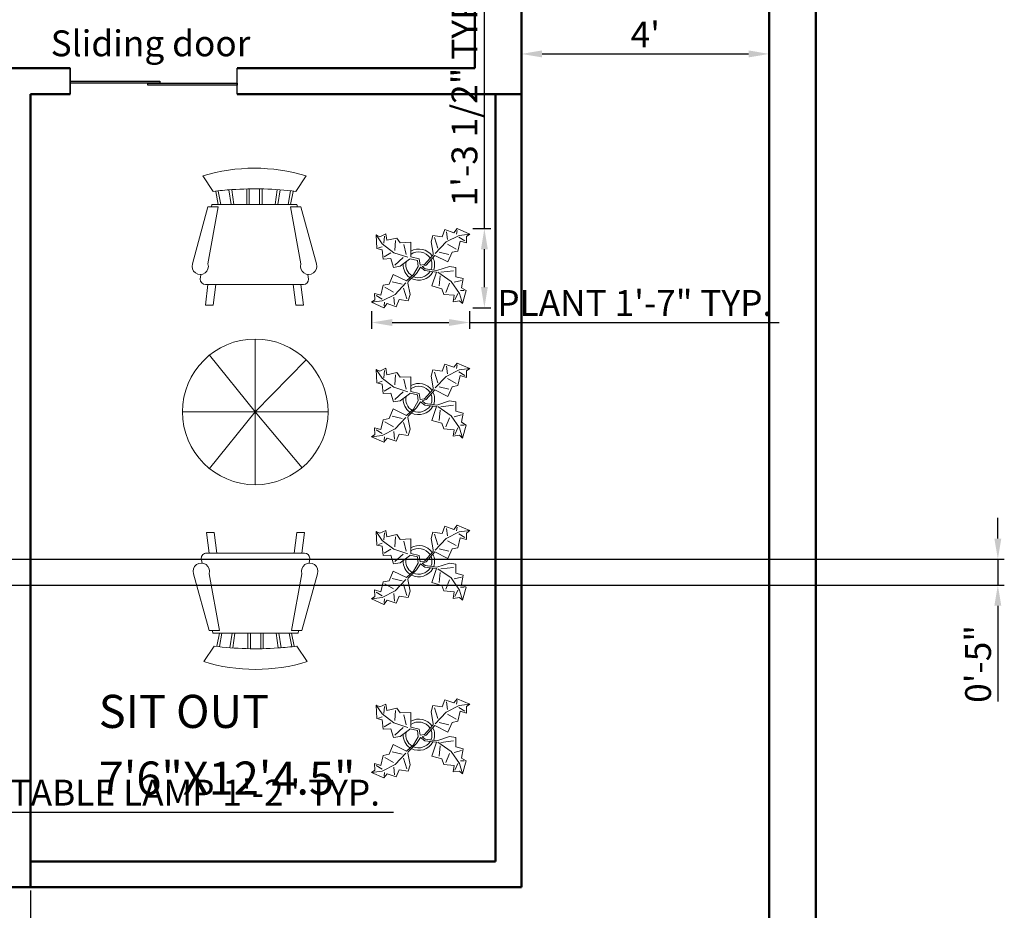
# Model space of a CAD drawing. Units: inches. Extents: x 116541 to 117938, y 135634 to 136328.
# Tile 7 of 9: x 117747 to 117938, y 135793 to 135965. Entities that reach past the tile are written whole.
import ezdxf

# ---------------------------------------------------------------- set-up
doc = ezdxf.new("R2010")
doc.units = ezdxf.units.IN
for name, color, linetype, lineweight in [('A-ANNO-DIMS', 2, 'Continuous', 18), ('A-ANNO-TEXT', 7, 'Continuous', 25), ('A-AREA-IDEN', 3, 'Continuous', 25), ('A-DOOR', 4, 'Continuous', 25), ('A-FURN', 8, 'Continuous', 18), ('A-WALL', 7, 'Continuous', 50)]:
    doc.layers.add(name, color=color, linetype=linetype, lineweight=lineweight)
doc.styles.get("Standard").update_dxf_attribs({"font": 'arial.ttf'})
doc.dimstyles.new('ISO-25', dxfattribs={"dimtxt": 5, "dimasz": 4, "dimexe": 1.25, "dimexo": 0.625, "dimtad": 1, "dimdec": 3, "dimlunit": 3, "dimtxsty": 'Standard', "dimcen": 2.5, "dimadec": 0, "dimazin": 0, "dimtfac": 1, "dimtdec": 3, "dimtmove": 0, "dimatfit": 3, "dimfxl": 1, "dimarcsym": 0})

# ---------------------------------------------------------------- blocks, each defined once
blk = doc.blocks.new('Chair - Rocking')
for p, q in [((-8, -4.5), (-10, -1.5)), ((8, -4.5), (10, -1.5)), ((-7.5, -4.5), (-7, -7)), ((-6.5, -7), (-7.02225, -4.43)), ((-4.5, -7), (-4.96674, -4.19951)), ((-4, -7), (-4.40532, -4.16272)), ((-1.5, -4.05012), (-1.5, -7)), ((-1, -7), (-1, -4.05012)), ((1, -7), (1, -4.04655)), ((1.5, -4.05012), (1.5, -7)), ((4, -7), (4.40187, -4.18694)), ((4.5, -7), (4.96761, -4.19437)), ((6.5, -7), (7, -4.4057)), ((7.5, -4.5), (7, -7)), ((-9, -7.5), (-12, -18.49999)), ((-7, -7.5), (-9, -7.5)), ((-9, -18.49999), (-7, -7.5)), ((-8.23428, -6.99939), (-8.3093, -7.47958)), ((-8.23041, -7), (8.23915, -7)), ((7, -7.5), (9, -7.5)), ((9, -18.49999), (7, -7.5)), ((8.31071, -7.48854), (8.23449, -7.00073)), ((9, -7.5), (12, -18.49999)), ((-10.36644, -20.64523), (-10.5, -21.49999)), ((10.5, -21.49999), (10.3575, -20.58798)), ((-9, -22.49999), (-9.5, -26.49999)), ((0, -22.49999), (-9.5, -22.49999)), ((-8, -26.49999), (-7.5, -22.49999)), ((0, -22.49999), (9.5, -22.49999)), ((8, -26.49999), (7.5, -22.49999)), ((9, -22.49999), (9.5, -26.49999)), ((-9.5, -26.49999), (-8, -26.49999)), ((9.5, -26.49999), (8, -26.49999))]:
    blk.add_line(p, q)
for centre, radius, start, end in [((0, -34.08333), 34.08333, 72.93847, 107.0615), ((0, -68.25004), 64.25, 93.92211, 97.15267), ((0, -68.25004), 64.25, 82.84733, 93.92211), ((-10.5, -18.99999), 1.58114, 161.5651, 18.43495), ((10.5, -18.99999), 1.58114, 161.5651, 18.43495), ((-9.5, -21.49999), 1, 180, 270), ((9.5, -21.49999), 1, 270, 0)]:
    blk.add_arc(centre, radius, start, end)
blk = doc.blocks.new('Plant - Rubber or Philodendron')
for p, q in [((-16.2005, 11.4774), (-13.9899, 8.1064)), ((-16.2005, 11.4774), (-14.8639, 10.7964)), ((-16.0159, 6.3329), (-16.2005, 11.4774)), ((-14.8639, 10.7964), (-12.6195, 11.8975)), ((-12.6195, 11.8975), (-12.1909, 9.4345)), ((4.6914, 8.8812), (5.3859, 11.2828)), ((5.3859, 11.2828), (8.8871, 10.7908)), ((8.8871, 10.7908), (9.9809, 13.4933)), ((9.9809, 13.4933), (13.3837, 12.301)), ((15.3859, 11.3055), (10.3916, 8.7942)), ((10.5828, 12.6946), (10.8893, 9.7953)), ((13.3837, 12.301), (14.68, 13.9039)), ((14.5816, 13.2037), (14.3848, 11.8033)), ((14.68, 13.9039), (19.3848, 11.8146)), ((19.3848, 11.8146), (15.3859, 11.3055)), ((19.3848, 11.8146), (18.1868, 10.9119)), ((-13.9899, 8.1064), (-9.5434, 4.7185)), ((-13.3174, 8.325), (-13.0735, 11.0065)), ((-12.1909, 9.4345), (-8.3829, 10.3)), ((-8.8369, 9.409), (-9.0894, 5.6095)), ((-8.3829, 10.3), (-7.0549, 8.501)), ((-7.0549, 8.501), (-3.0284, 8.6941)), ((-4.8529, 4.012), (-5.7184, 7.82)), ((-3.0284, 8.6941), (-3.0709, 3.1041)), ((4.6914, 8.8812), (5.5014, 4.4831)), ((5.9878, 10.4842), (7.1971, 6.3869)), ((10.3916, 8.7942), (6.2847, 4.4028)), ((14.2977, 6.1031), (10.9934, 7.9956)), ((15.7909, 9.1065), (14.8995, 5.3044)), ((15.2875, 10.6053), (17.5907, 9.2105)), ((18.1925, 8.4119), (15.7909, 9.1065)), ((18.1868, 10.9119), (18.1925, 8.4119)), ((-14.0069, 5.8704), (-16.0159, 6.3329)), ((-15.3434, 6.5514), (-13.9984, 6.9884)), ((-13.5868, 2.2894), (-14.0069, 5.8704)), ((-13.1329, 3.1804), (-10.6614, 4.727)), ((-9.5434, 4.7185), (-4.1917, 2.9888)), ((2.1141, 0.2298), (5.4346, 3.9146)), ((5.4346, 3.9146), (5.5014, 4.4831)), ((7.7005, 4.8881), (11.5025, 3.9967)), ((12.7005, 4.8994), (11.1089, 1.1958)), ((14.8995, 5.3044), (12.7005, 4.8994)), ((-10.6784, 2.491), (-13.5868, 2.2894)), ((-9.5858, -0.8715), (-10.6784, 2.491)), ((-9.1318, 0.0195), (-5.9793, 2.9025)), ((-7.1228, -0.443), (-3.5248, 2.2131)), ((-3.5248, 2.2131), (-3.3011, 2.4355)), ((-3.3011, 2.4355), (-0.5306, 1.7947)), ((-3.0709, 3.1041), (0.0797, 2.3163)), ((-0.5306, 1.7947), (-0.2255, -0.5527)), ((-0.5306, 1.7947), (-0.5306, 1.7947)), ((0.0797, 2.3163), (0.4866, -0.031)), ((0.4866, -0.031), (2.1141, 0.2298)), ((6.1032, 3.6844), (2.8262, -0.031)), ((11.1089, 1.1958), (6.1032, 3.6844)), ((-11.3237, -7.2629), (-9.7321, -3.5593)), ((-9.7321, -3.5593), (-4.7264, -6.0479)), ((-7.1228, -0.443), (-9.5858, -0.8715)), ((-2.019, -3.6148), (-4.7264, -6.0479)), ((-4.0579, -6.2781), (-0.9375, -3.1608)), ((-2.019, -3.6148), (-0.2255, -0.5527)), ((-0.9375, -3.1608), (0.5883, -0.8135)), ((0.5883, -0.8135), (2.2447, -2.0916)), ((2.8262, -0.031), (1.3003, -0.5527)), ((1.3003, -0.5527), (2.4193, -1.4655)), ((2.2447, -2.0916), (6.7108, -2.6626)), ((2.4193, -1.4655), (6.895, -2.1175)), ((4.943, -7.9659), (6.7108, -2.6626)), ((11.6605, -0.5413), (6.895, -2.1175)), ((12.3677, -6.1981), (7.219, -2.6772)), ((8.3544, -2.7453), (13.1973, -2.1704)), ((11.6605, -0.5413), (14.1354, -0.8948)), ((14.1354, -0.8948), (14.1354, -4.4304)), ((-13.5228, -7.6679), (-11.3237, -7.2629)), ((-6.3237, -7.2516), (-10.1257, -6.3602)), ((-9.0148, -11.1577), (-4.9047, -6.8122)), ((-4.1246, -6.8466), (-4.0579, -6.2781)), ((-3.3146, -11.2447), (-4.1246, -6.8466)), ((8.125, -4.0768), (7.7715, -7.9659)), ((10.2463, -10.4408), (11.6605, -6.9053)), ((15.5496, -10.7943), (12.3677, -6.1981)), ((16.2567, -5.8446), (13.4283, -6.5517)), ((14.1354, -4.4304), (16.9638, -5.1375)), ((16.9638, -5.1375), (16.2567, -8.673)), ((-16.8157, -10.7754), (-14.4141, -11.4699)), ((-16.8101, -13.2754), (-16.8157, -10.7754)), ((-14.4141, -11.4699), (-13.5228, -7.6679)), ((-14.0091, -13.669), (-9.0148, -11.1577)), ((-12.921, -8.4665), (-9.6166, -10.359)), ((-4.611, -12.8477), (-5.8203, -8.7504)), ((-3.3146, -11.2447), (-4.0092, -13.6463)), ((8.8321, -9.0266), (4.943, -7.9659)), ((9.5392, -11.1479), (8.8321, -9.0266)), ((13.4283, -11.5015), (9.5392, -11.1479)), ((14.8425, -10.7943), (13.7819, -13.2692)), ((16.6103, -14.6834), (15.5496, -10.7943)), ((17.3174, -9.7337), (15.9032, -9.7337)), ((16.2567, -8.673), (18.0245, -9.7337)), ((18.0245, -9.7337), (16.6103, -14.6834)), ((-18.008, -14.1781), (-16.8101, -13.2754)), ((-18.008, -14.1781), (-14.0091, -13.669)), ((-13.3032, -16.2674), (-18.008, -14.1781)), ((-13.9107, -12.9688), (-16.2139, -11.574)), ((-12.0069, -14.6645), (-13.3032, -16.2674)), ((-13.2048, -15.5672), (-13.008, -14.1668)), ((-8.6042, -15.8568), (-12.0069, -14.6645)), ((-9.206, -15.0581), (-9.5126, -12.1588)), ((-7.5103, -13.1543), (-8.6042, -15.8568)), ((-4.0092, -13.6463), (-7.5103, -13.1543)), ((13.0748, -13.9763), (13.4283, -11.5015)), ((15.5496, -13.6228), (13.0748, -13.9763)), ((16.6103, -14.6834), (15.5496, -13.6228))]:
    blk.add_line(p, q)
for centre, radius, start, end in [((0, 0), 6.1275, 34.37569, 120.1028), ((-0.0601, -0.2075), 5.2461, 33.82192, 124.9414), ((0.0308, 0.1664), 6, 178.6147, 235.1169), ((0.0308, 0.1664), 5, 168.1647, 238.6725), ((-0.2664, 0.1682), 5.2775, 338.4094, 20.03007), ((-0.098, 0.1364), 6.1288, 341.2017, 26.09184), ((-0.0234, 0.3825), 6.1492, 242.5812, 331.2714), ((-0.1102, 0.4886), 5.2883, 247.3711, 327.472)]:
    blk.add_arc(centre, radius, start, end)
blk = doc.blocks.new('*D50')
at = {"layer": 'A-ANNO-DIMS', "color": 0, "lineweight": -2, "transparency": 16777216}
for p, q in [((117487.52, 135796.88), (117487.52, 135773.9)), ((117749.52, 135796.88), (117749.52, 135773.9)), ((117491.52, 135775.15), (117745.52, 135775.15))]:
    blk.add_line(p, q, dxfattribs=at)
at = {"layer": 'A-ANNO-DIMS', "color": 0, "transparency": 16777216}
for points in [[(117491.52, 135775.82), (117491.52, 135774.49), (117487.52, 135775.15)], [(117745.52, 135775.82), (117745.52, 135774.49), (117749.52, 135775.15)]]:
    blk.add_solid(points, dxfattribs=at)
at = {"layer": 'Defpoints', "color": 0, "transparency": 16777216}
for p in [(117487.52, 135797.5), (117749.52, 135797.5), (117749.52, 135775.15)]:
    blk.add_point(p, dxfattribs=at)
at = {"layer": 'A-ANNO-DIMS', "color": 0, "transparency": 16777216, "insert": (117618.52, 135778.33), "char_height": 5, "attachment_point": 5}
blk.add_mtext('21\'-10"', dxfattribs=at)
blk = doc.blocks.new('*D51')
at = {"layer": 'A-ANNO-DIMS', "color": 0, "lineweight": -2, "transparency": 16777216}
for p, q in [((117844.52, 135951.63), (117844.52, 135960.04)), ((117892.52, 135951.63), (117892.52, 135960.04)), ((117848.52, 135958.79), (117888.52, 135958.79))]:
    blk.add_line(p, q, dxfattribs=at)
at = {"layer": 'A-ANNO-DIMS', "color": 0, "transparency": 16777216}
for points in [[(117848.52, 135959.46), (117848.52, 135958.12), (117844.52, 135958.79)], [(117888.52, 135959.46), (117888.52, 135958.12), (117892.52, 135958.79)]]:
    blk.add_solid(points, dxfattribs=at)
at = {"layer": 'Defpoints', "color": 0, "transparency": 16777216}
for p in [(117892.52, 135958.79), (117844.52, 135951), (117892.52, 135951)]:
    blk.add_point(p, dxfattribs=at)
at = {"layer": 'A-ANNO-DIMS', "color": 0, "transparency": 16777216, "insert": (117868.52, 135961.91), "char_height": 5, "attachment_point": 5}
blk.add_mtext("4'", dxfattribs=at)
blk = doc.blocks.new('*D60')
at = {"layer": 'A-ANNO-DIMS', "color": 0, "lineweight": -2, "transparency": 16777216}
for p, q in [((117815.51, 135909.03), (117815.51, 135905.56)), ((117834.51, 135909.03), (117834.51, 135905.56)), ((117819.51, 135906.81), (117830.51, 135906.81)), ((117834.51, 135906.81), (117894.45, 135906.81))]:
    blk.add_line(p, q, dxfattribs=at)
at = {"layer": 'A-ANNO-DIMS', "color": 0, "transparency": 16777216}
for points in [[(117819.51, 135907.47), (117819.51, 135906.14), (117815.51, 135906.81)], [(117830.51, 135907.47), (117830.51, 135906.14), (117834.51, 135906.81)]]:
    blk.add_solid(points, dxfattribs=at)
at = {"layer": 'Defpoints', "color": 0, "transparency": 16777216}
for p in [(117815.51, 135909.66), (117834.51, 135909.66), (117834.51, 135906.81)]:
    blk.add_point(p, dxfattribs=at)
at = {"layer": 'A-ANNO-DIMS', "color": 0, "transparency": 16777216, "insert": (117866.48, 135909.94), "char_height": 5, "attachment_point": 5}
blk.add_mtext('PLANT 1\'-7" TYP.', dxfattribs=at)
blk = doc.blocks.new('*D61')
at = {"layer": 'A-ANNO-DIMS', "color": 0, "lineweight": -2, "transparency": 16777216}
for p, q in [((117837.36, 135924.99), (117837.36, 135971.9)), ((117835.14, 135924.99), (117838.61, 135924.99)), ((117837.36, 135913.66), (117837.36, 135920.99)), ((117835.14, 135909.66), (117838.61, 135909.66))]:
    blk.add_line(p, q, dxfattribs=at)
at = {"layer": 'A-ANNO-DIMS', "color": 0, "transparency": 16777216}
for points in [[(117836.7, 135920.99), (117838.03, 135920.99), (117837.36, 135924.99)], [(117836.7, 135913.66), (117838.03, 135913.66), (117837.36, 135909.66)]]:
    blk.add_solid(points, dxfattribs=at)
at = {"layer": 'Defpoints', "color": 0, "transparency": 16777216}
for p in [(117834.51, 135924.99), (117837.36, 135924.99), (117834.51, 135909.66)]:
    blk.add_point(p, dxfattribs=at)
at = {"layer": 'A-ANNO-DIMS', "color": 0, "transparency": 16777216, "insert": (117834.15, 135950.44), "char_height": 5, "attachment_point": 5, "rotation": 90}
blk.add_mtext('1\'-3 1/2" TYP.', dxfattribs=at)
blk = doc.blocks.new('*D68')
at = {"layer": 'A-ANNO-DIMS', "color": 0, "lineweight": -2, "transparency": 16777216}
for p, q in [((117724.85, 135813.5), (117724.85, 135810.78)), ((117738.85, 135813.5), (117738.85, 135810.78)), ((117728.85, 135812.03), (117734.85, 135812.03)), ((117738.85, 135812.03), (117819.74, 135812.03))]:
    blk.add_line(p, q, dxfattribs=at)
at = {"layer": 'A-ANNO-DIMS', "color": 0, "transparency": 16777216}
for points in [[(117728.85, 135812.7), (117728.85, 135811.36), (117724.85, 135812.03)], [(117734.85, 135812.7), (117734.85, 135811.36), (117738.85, 135812.03)]]:
    blk.add_solid(points, dxfattribs=at)
at = {"layer": 'Defpoints', "color": 0, "transparency": 16777216}
for p in [(117724.85, 135814.13), (117738.85, 135814.13), (117738.85, 135812.03)]:
    blk.add_point(p, dxfattribs=at)
at = {"layer": 'A-ANNO-DIMS', "color": 0, "transparency": 16777216, "insert": (117781.3, 135815.17), "char_height": 5, "attachment_point": 5}
blk.add_mtext('TABLE LAMP 1\'-2" TYP.', dxfattribs=at)
blk = doc.blocks.new('*D104')
at = {"layer": 'A-ANNO-DIMS', "color": 0, "lineweight": -2, "transparency": 16777216}
for p, q in [((117936.77, 135865), (117936.77, 135869)), ((117526.85, 135861), (117938.02, 135861)), ((117936.77, 135861), (117936.77, 135856)), ((117526.85, 135856), (117938.02, 135856)), ((117936.77, 135852), (117936.77, 135833.46))]:
    blk.add_line(p, q, dxfattribs=at)
at = {"layer": 'A-ANNO-DIMS', "color": 0, "transparency": 16777216}
for points in [[(117936.1, 135865), (117937.44, 135865), (117936.77, 135861)], [(117936.1, 135852), (117937.44, 135852), (117936.77, 135856)]]:
    blk.add_solid(points, dxfattribs=at)
at = {"layer": 'Defpoints', "color": 0, "transparency": 16777216}
for p in [(117526.22, 135861), (117526.22, 135856), (117936.77, 135856)]:
    blk.add_point(p, dxfattribs=at)
at = {"layer": 'A-ANNO-DIMS', "color": 0, "transparency": 16777216, "insert": (117933.59, 135840.73), "char_height": 5, "attachment_point": 5, "rotation": 90}
blk.add_mtext('0\'-5"', dxfattribs=at)

msp = doc.modelspace()

# ---------------------------------------------------------------- linework, layer by layer
at = {"layer": 'A-DOOR'}
msp.add_line((117789.5261, 135951.0034), (117789.5261, 135956.0034), dxfattribs=at)
for points in [[(117757.1864, 135951.0034), (117757.1864, 135951.0034), (117757.1864, 135956.0034), (117757.1864, 135956.0034)], [(117757.1864, 135953.5034), (117774.5199, 135953.5034), (117774.5199, 135953.1219), (117757.1864, 135953.1219)], [(117772.1926, 135953.1219), (117789.5261, 135953.1219), (117789.5261, 135952.7404), (117772.1926, 135952.7404)]]:
    msp.add_lwpolyline(points, close=True, dxfattribs=at)
at = {"layer": 'A-FURN'}
for q in [(117793.0025, 135903.6107), (117784.1711, 135900.5019), (117802.8413, 135899.6098), (117778.9044, 135889.5127), (117784.1545, 135878.5369), (117793.0025, 135875.4147), (117807.1005, 135889.5127), (117802.0564, 135878.7062)]:
    msp.add_line((117793.0025, 135889.5127), q, dxfattribs=at)
msp.add_circle((117793.0025, 135889.5127), 14.098, dxfattribs=at)
at = {"layer": 'A-WALL'}
for p, q in [((117901.5209, 136286.5034), (117901.5209, 135734.5034)), ((117844.5209, 135951.0034), (117844.5209, 136253.5034)), ((117892.5209, 136244.5034), (117892.5209, 135750.0323)), ((117835.5209, 135956.0034), (117835.5209, 136077.5034)), ((117735.0567, 135956.0034), (117757.1864, 135956.0034)), ((117789.5261, 135956.0034), (117835.5209, 135956.0034)), ((117844.5209, 135956.0034), (117844.5209, 135802.5034)), ((117749.5209, 135951.0034), (117749.5209, 135797.5034)), ((117749.5209, 135951.0034), (117757.1864, 135951.0034)), ((117789.5261, 135951.0034), (117844.5209, 135951.0034)), ((117839.5209, 135951.0034), (117839.5209, 135802.5034)), ((117749.5209, 135802.5034), (117839.5209, 135802.5034)), ((117844.5209, 135802.5034), (117844.5209, 135797.5034)), ((117487.5209, 135797.5034), (117749.5209, 135797.5034)), ((117749.5209, 135797.5034), (117844.5209, 135797.5034))]:
    msp.add_line(p, q, dxfattribs=at)

# ---------------------------------------------------------------- block references
at = {"layer": 'A-FURN'}
msp.add_blockref('Chair - Rocking', (117792.8425, 135936.6724), dxfattribs=at)
at = {"layer": 'A-FURN', "xscale": 0.50815865363942, "yscale": 0.50815865363942, "zscale": 0.50815865363942}
for p in [(117824.6642, 135917.9221), (117824.6642, 135891.8975), (117824.6642, 135860.5201), (117824.6642, 135826.928)]:
    msp.add_blockref('Plant - Rubber or Philodendron', p, dxfattribs=at)
at = {"layer": 'A-FURN', "rotation": 180}
msp.add_blockref('Chair - Rocking', (117793.0502, 135839.6701), dxfattribs=at)

# ---------------------------------------------------------------- texts
at = {"layer": 'A-ANNO-TEXT', "insert": (117753.3944, 135963.3389), "char_height": 5, "attachment_point": 1}
msp.add_mtext_dynamic_manual_height_columns('{\\fArial|b1|i0|c0|p34;Sliding door}', width=154.753188, gutter_width=166.7036, heights=[0], dxfattribs=at)
at = {"layer": 'A-AREA-IDEN'}
for s, height, p in [('SIT OUT', 6.40837, (117762.6991, 135828.3386)), ('7\'6"X12\'4.5"', 6.408368, (117762.6991, 135815.4293))]:
    msp.add_text(s, height=height, dxfattribs=at).set_placement(p)

# ---------------------------------------------------------------- dimensions: what is measured, and where the dimension line sits
at = {"layer": 'A-ANNO-DIMS'}
dim = msp.add_linear_dim(base=(117837.365, 135924.9875), p1=(117834.5148, 135909.6557), p2=(117834.5148, 135924.9875), angle=90, text='<> TYP.', dimstyle='ISO-25', override={"dimdec": 1, "dimrnd": 0, "dimzin": 1, "dimlunit": 4, "dimfrac": 2}, dxfattribs=at)
dim.commit()
dim.dimension.update_dxf_attribs({"geometry": '*D61', "text_midpoint": (117834.153, 135950.4413)})
for base, p1, p2, picture, middle in [((117892.5209, 135958.7891), (117844.5209, 135951.0034), (117892.5209, 135951.0034), '*D51', (117868.5209, 135961.9141)), ((117749.5209, 135775.1534), (117487.5209, 135797.5034), (117749.5209, 135797.5034), '*D50', (117618.5209, 135778.3313))]:
    dim = msp.add_linear_dim(base=base, p1=p1, p2=p2, dimstyle='ISO-25', override={"dimclrd": 0, "dimclre": 0, "dimclrt": 0}, dxfattribs=at)
    dim.commit()
    dim.dimension.update_dxf_attribs({"geometry": picture, "text_midpoint": middle})
for base, p1, p2, text, picture, middle in [((117834.5148, 135906.8054), (117815.5133, 135909.6557), (117834.5148, 135909.6557), 'PLANT <> TYP.', '*D60', (117866.4812, 135909.9424)), ((117738.853, 135812.0291), (117724.853, 135814.1291), (117738.853, 135814.1291), 'TABLE LAMP <> TYP.', '*D68', (117781.2952, 135815.166))]:
    dim = msp.add_linear_dim(base=base, p1=p1, p2=p2, text=text, dimstyle='ISO-25', override={"dimdec": 1, "dimrnd": 0, "dimzin": 1, "dimlunit": 4, "dimfrac": 2}, dxfattribs=at)
    dim.commit()
    dim.dimension.update_dxf_attribs({"geometry": picture, "text_midpoint": middle})
dim = msp.add_linear_dim(base=(117936.7709, 135856.0034), p1=(117526.2247, 135861.0034), p2=(117526.2247, 135856.0034), angle=90, dimstyle='ISO-25', override={"dimdec": 1, "dimlfac": 1, "dimrnd": 0, "dimzin": 1, "dimdsep": 46, "dimlunit": 4, "dimfrac": 2}, dxfattribs=at)
dim.commit()
dim.dimension.update_dxf_attribs({"geometry": '*D104', "text_midpoint": (117933.593, 135840.7328)})

doc.saveas('drawing.dxf')
